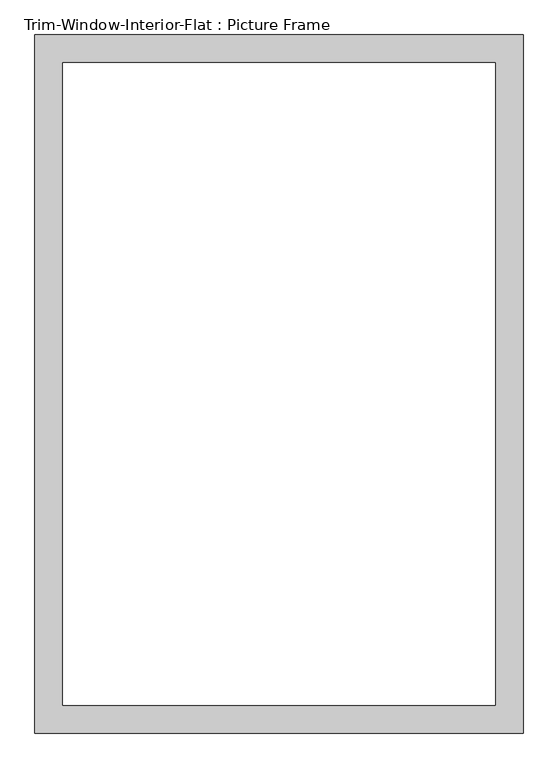
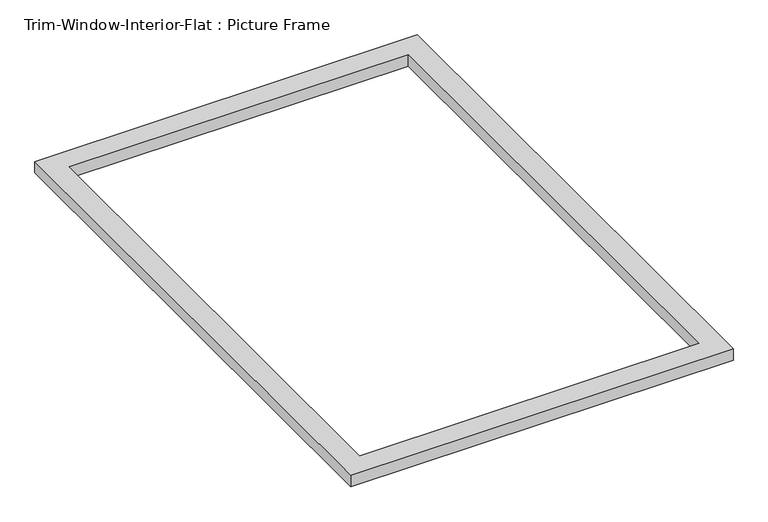
"""IFC4 building model written with IfcOpenShell, lengths in millimetres: proxy geometry, Trim-Window-Interior-Flat : Picture Frame."""

from ifc_helpers import new_model, si_unit, origin, origin_with_axes, place, context, project, spatial, polyline, outline, extrude, source, transform, mapped, element, save


def trim_window_interior_flat_picture_frame_d5b7f3a4(model_context):
    return source(origin(), model_context, "Body", "SweptSolid", [
        extrude(outline(polyline([(501.65, 44.45), (501.65, -1390.65), (-501.65, -1390.65), (-501.65, 44.45), (501.65, 44.45)]), holes=[polyline([(444.5, -12.7), (-444.5, -12.7), (-444.5, -1333.5), (444.5, -1333.5), (444.5, -12.7)])]), origin_with_axes(), (0.0, 0.0, 1.0), 31.75),
    ])


if __name__ == "__main__":
    model = new_model("IFC4")
    model_context = context("Model", 3, world=origin())
    ifc_project = project(units=[si_unit("LENGTHUNIT", "METRE", prefix="MILLI")], contexts=[model_context])
    site = spatial("IfcSite", under=ifc_project)
    building = spatial("IfcBuilding", under=site)
    placement = place(None, origin())
    trim_window_interior_flat_picture_frame_shape = trim_window_interior_flat_picture_frame_d5b7f3a4(model_context)
    element("IfcBuildingElementProxy", 1, Name="Trim-Window-Interior-Flat : Picture Frame", ObjectType="Trim-Window-Interior-Flat : Picture Frame", at=placement, inside=building, context=model_context, shape_type="MappedRepresentation", body=[
        mapped(trim_window_interior_flat_picture_frame_shape, transform((0.0, 0.0, 0.0), x_axis=(1.0, 0.0, 0.0), y_axis=(0.0, 1.0, 0.0), z_axis=(0.0, 0.0, 1.0))),
    ])
    save(model, "model.ifc")

# Revit data of these elements
# Type "Trim-Window-Interior-Flat : Picture Frame"
#   Trim Thickness_Picture Frame = 0' - 1 1/4"
#   Trim Width = 0' - 2 1/4"
#   Trim Thickness_with Sill = 0' - 0 3/4"
#   Sill Thickness = 0' - 1 1/4"
#   Opening Width [instance default] = 2' - 0"
#   Opening Height [instance default] = 3' - 0"
#   Default Elevation = 4' - 0"
#   Sill = no
#   Picture Frame = yes
#   Trim Material [instance default] = none
# Element 1 (IfcBuildingElementProxy, "Trim-Window-Interior-Flat : Picture Frame")
#   Opening Width = 3' - 0"
#   Opening Height = 4' - 5"
#   Trim Material = Wood - Stained
#   Materials on its faces: "Wood - Stained"
# Materials
#   "Wood - Stained": class "Wood", colour RGB 224 178 126, transparency 0, Cost = 0
